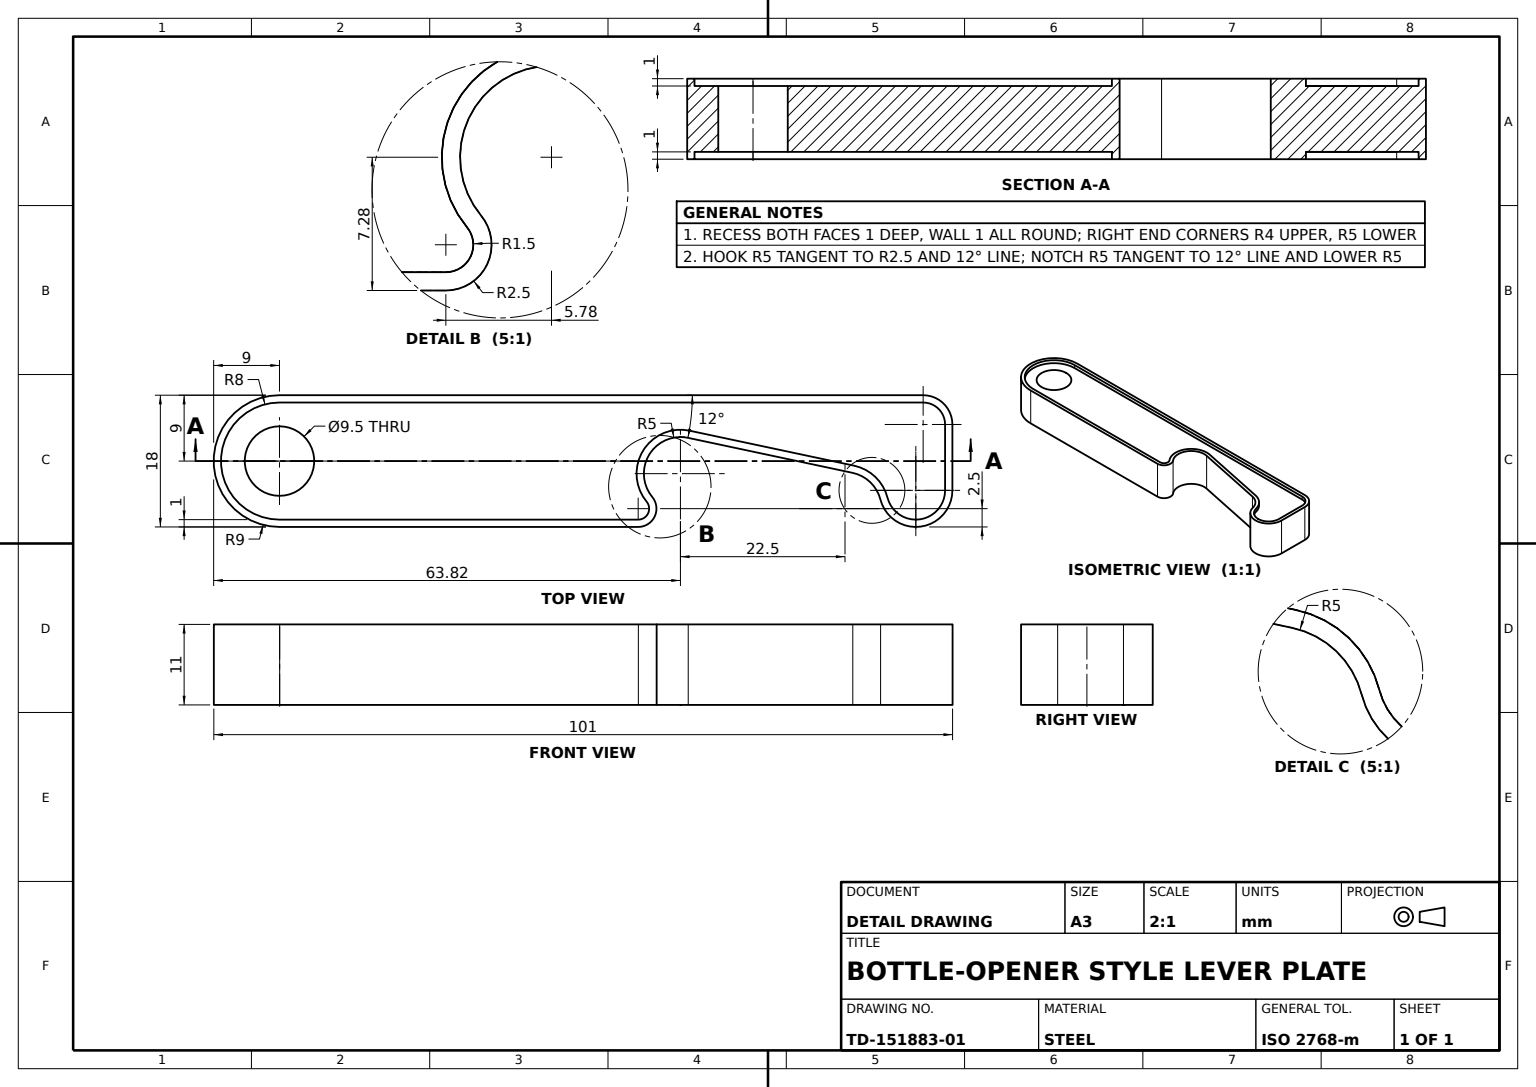
SolidWorks part; units mm, degrees
material "Plain Carbon Steel"
ref_plane "Front Plane" through (0, 0, 0) normal (0, 0, 1) x (1, 0, 0)
ref_plane "Top Plane" through (0, 0, 0) normal (0, 1, 0) x (1, 0, 0)
ref_plane "Right Plane" through (0, 0, 0) normal (1, 0, 0) x (0, 0, -1)
sketch "Lever Profile Sketch" plane through (0, 0, 0) normal (0, 1, 0) x (1, 0, 0)
  line L1 (46.5, 9) -> (-41.5, 9)
  line L2 (50.5, 5) -> (50.5, -4)
  line L3 (7.5402, -9) -> (-41.5, -9)
  line L6 (14.3571, 3.1733) -> (36.8571, -1.6093)
  arc A0 (46.5, 9) -> (50.5, 5) centre (46.5, 5) cw
  arc A1 (40.6588, -5.25) -> (50.5, -4) centre (45.5, -4) ccw
  circle A2 centre (-41.5, 0) radius 4.75
  arc A3 (-41.5, 9) -> (-41.5, -9) centre (-41.5, 0) ccw
  arc A5 (40.6588, -5.25) -> (36.8571, -1.6093) centre (35.8175, -6.5) ccw
  arc A6 (14.3571, 3.1733) -> (9.466, -4.9058) centre (13.3175, -1.7175) ccw
  arc A7 (7.5402, -9) -> (9.466, -4.9058) centre (7.5402, -6.5) ccw
  point P0 (0, 0)
  point P16 (50.5, -6.5)
  point P18 (-50.5, -6.5)
  dimension "D3" = 4
  dimension "D4" = 10
  dimension "D5" = 18
  dimension "D6" = 9.5
  dimension "D7" = 12
  dimension "D8" = 22.5
  dimension "D9" = 10
  dimension "D10" = 5
  dimension "D11" = 5
  dimension "D13" = 50.5
  dimension "D2" = 5
  dimension "D12" = 9.8412
  dimension "D14" = 92
extrude "Lever Body 11mm" add sketch "Lever Profile Sketch" along normal mid plane 11
sketch "Face Recess Sketch" plane through (0, 5.5, 0) normal (0, 1, 0) x (1, 0, 0)
  line L8 (-41.5, -8) -> (7.5402, -8)
  line L9 (14.565, 4.1514) -> (37.065, -0.6311)
  line L10 (49.5, -4) -> (49.5, 5)
  line L11 (46.5, 8) -> (-41.5, 8)
  line L12 (-41.5, -8) -> (7.5402, -8)
  line L13 (14.565, 4.1514) -> (37.065, -0.6311)
  line L14 (49.5, -4) -> (49.5, 5)
  line L15 (46.5, 8) -> (-41.5, 8)
  arc A12 (-41.5, 8) -> (-41.5, -8) centre (-41.5, 0) ccw
  arc A13 (7.5402, -8) -> (8.6957, -5.5435) centre (7.5402, -6.5) ccw
  arc A14 (14.565, 4.1514) -> (8.6957, -5.5435) centre (13.3175, -1.7175) ccw
  arc A15 (41.627, -5) -> (37.065, -0.6311) centre (35.8175, -6.5) ccw
  arc A16 (41.627, -5) -> (49.5, -4) centre (45.5, -4) ccw
  arc A17 (49.5, 5) -> (46.5, 8) centre (46.5, 5) ccw
  arc A18 (-41.5, 8) -> (-41.5, -8) centre (-41.5, 0) ccw
  arc A19 (7.5402, -8) -> (8.6957, -5.5435) centre (7.5402, -6.5) ccw
  arc A20 (14.565, 4.1514) -> (8.6957, -5.5435) centre (13.3175, -1.7175) ccw
  arc A21 (41.627, -5) -> (37.065, -0.6311) centre (35.8175, -6.5) ccw
  arc A22 (41.627, -5) -> (49.5, -4) centre (45.5, -4) ccw
  arc A23 (49.5, 5) -> (46.5, 8) centre (46.5, 5) ccw
  dimension "D1" = 1
extrude "Top Face Recess 1mm" cut sketch "Face Recess Sketch" against normal blind 1
mirror "Bottom Face Recess Mirror" about plane through (0, 0, 0) normal (0, 1, 0) of "Top Face Recess 1mm"
